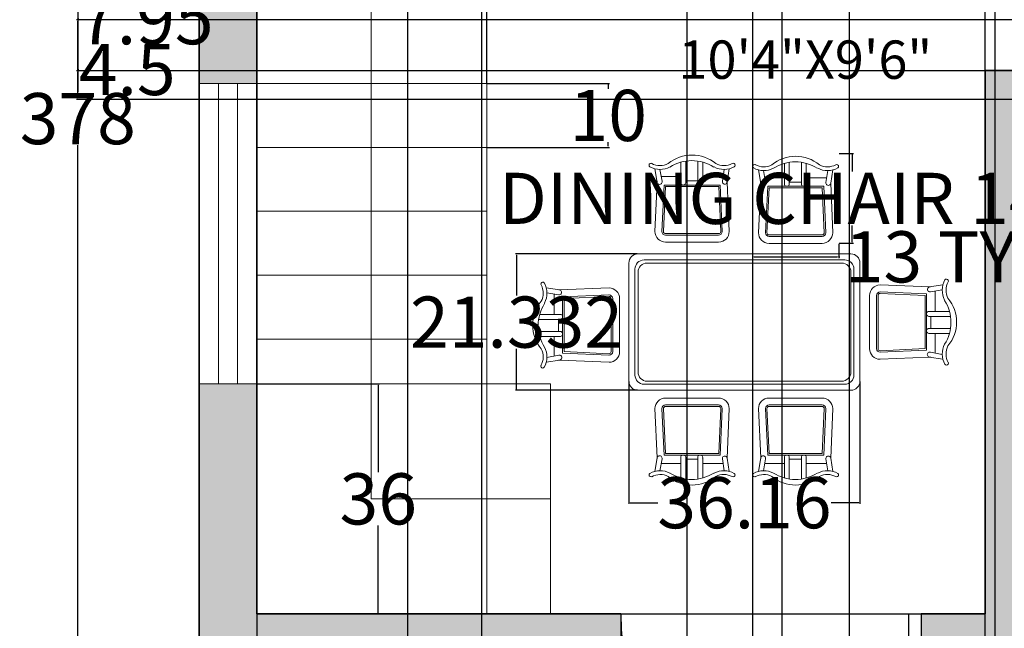
# Model space of a CAD drawing. Units: inches. Extents: x -24 to 368, y -370 to 58.
# Tile 2 of 9: x -24 to 130, y -235 to -140. Entities that reach past the tile are written whole.
import ezdxf

# ---------------------------------------------------------------- set-up
doc = ezdxf.new("R2010")
doc.units = ezdxf.units.IN
doc.header["$MEASUREMENT"] = 0
for name, color, linetype, lineweight in [('A-ANNO-DIMS', 2, 'Continuous', 18), ('A-AREA-IDEN', 7, 'Continuous', 18), ('A-FLOR-STRS', 7, 'Continuous', 18), ('A-WALL', 7, 'Continuous', 35), ('Furniture', 7, 'Continuous', 15)]:
    doc.layers.add(name, color=color, linetype=linetype, lineweight=lineweight)
for name, color, linetype, lineweight, true_color in [('A-DOOR', 40, 'Continuous', 25, 0xf8d731), ('A-GLAZ', 30, 'Continuous', 18, 0xf26722), ('A-WALL-PATT', 18, 'Continuous', 13, 0x000000)]:
    doc.layers.add(name, color=color, linetype=linetype, lineweight=lineweight, true_color=true_color)
doc.styles.get("Standard").update_dxf_attribs({"font": 'arial.ttf'})
doc.dimstyles.get("Standard").update_dxf_attribs({"dimtxt": 8, "dimasz": 0.18, "dimexe": 0.18, "dimexo": 0.0625, "dimgap": 0.09, "dimtad": 0, "dimtih": 1, "dimtoh": 1, "dimdec": 4, "dimzin": 0, "dimdsep": 46, "dimlunit": 3, "dimtxsty": 'Standard', "dimcen": 0.09, "dimclre": 5, "dimclrt": 6, "dimadec": 0, "dimazin": 0, "dimtfac": 1, "dimtdec": 4, "dimtofl": 0, "dimtmove": 0, "dimatfit": 3, "dimfxl": 1, "dimtolj": 1, "dimtzin": 0, "dimarcsym": 0})

# ---------------------------------------------------------------- blocks, each defined once
blk = doc.blocks.new('CHAIR-DINING')
for p, q in [((4.98, 9.38), (4.98, 12.51)), ((5.74, 9.38), (5.74, 12.67)), ((7.64, 12.68), (7.64, 9.38)), ((8.4, 12.52), (8.4, 9.39)), ((1.28, 9.34), (0.93, 11.48)), ((2.04, 9.52), (1.69, 11.38)), ((11.79, 11.38), (11.48, 9.52)), ((12.55, 11.48), (12.24, 9.4)), ((0.93, 1.66), (1.28, 9.34)), ((1.9, 10.25), (4.98, 10.25)), ((5.74, 9.59), (7.64, 9.59)), ((8.4, 10.25), (11.6, 10.25)), ((12.24, 9.4), (12.55, 1.66)), ((2.02, 1.67), (2.37, 8.93)), ((2.26, 1.66), (2.6, 8.69)), ((2.37, 8.93), (11.15, 8.93)), ((2.6, 8.69), (10.92, 8.69)), ((10.92, 8.69), (11.22, 1.66)), ((11.15, 8.93), (11.46, 1.67)), ((10.89, 1.33), (2.59, 1.33)), ((10.89, 1.09), (2.59, 1.09)), ((10.89, 0), (2.59, 0))]:
    blk.add_line(p, q)
for centre, radius, start, end in [((0.3, 12.04), 0.297, 56.5726, 237.7215), ((6.74, 7.78), 5.84, 50.3459, 129.6541), ((6.7, 6.41), 6.34, 57.3186, 122.6814), ((13.18, 12.04), 0.297, 302.2785, 123.4274), ((1.75, 14.71), 3.33, 241.1173, 297.5141), ((1.75, 14.71), 2.74, 240.9211, 297.5141), ((11.73, 14.71), 3.33, 242.4859, 298.8827), ((11.73, 14.71), 2.74, 242.4859, 298.022), ((1.66, 9.43), 0.39, 166.2748, 13.7252), ((5.36, 9.31), 0.387, 168.6748, 11.3252), ((8.02, 9.31), 0.387, 168.8014, 12.2085), ((11.86, 9.46), 0.384, 170.8614, 9.1386), ((2.59, 1.66), 1.66, 180, 270), ((2.59, 1.66), 0.569, 180, 270), ((2.59, 1.66), 0.332, 180, 270), ((10.89, 1.66), 1.66, 270, 0), ((10.89, 1.66), 0.569, 270, 0), ((10.89, 1.66), 0.332, 270, 0)]:
    blk.add_arc(centre, radius, start, end)
blk = doc.blocks.new('WINDOW-47')
for p, q in [((0, 47), (0, 0)), ((0, 47), (9, 47)), ((3, 47), (3, 0)), ((6, 47), (6, 0)), ((9, 0), (9, 47)), ((0, 0), (9, 0))]:
    blk.add_line(p, q)
blk = doc.blocks.new('DOOR-SINGLE-47')
for p, q in [((0, 0), (0, 47)), ((2, 0), (2, 47)), ((47, 0), (0, 0))]:
    blk.add_line(p, q)
blk.add_arc((0, 0), 47, 0, 90)
blk = doc.blocks.new('*D11')
at = {"layer": 'A-ANNO-DIMS', "color": 5, "lineweight": -2, "transparency": 16777216}
for p, q in [((104.31, -160.81), (106.54, -160.81)), ((104.31, -174.87), (106.54, -174.87))]:
    blk.add_line(p, q, dxfattribs=at)
at = {"layer": 'A-ANNO-DIMS', "color": 0, "lineweight": -2, "transparency": 16777216}
for p, q in [((106.36, -160.99), (106.36, -163.61)), ((106.36, -174.69), (106.36, -172.07))]:
    blk.add_line(p, q, dxfattribs=at)
at = {"layer": 'A-ANNO-DIMS', "color": 0, "transparency": 16777216}
for points in [[(106.33, -160.99), (106.39, -160.99), (106.36, -160.81)], [(106.33, -174.69), (106.39, -174.69), (106.36, -174.87)]]:
    blk.add_solid(points, dxfattribs=at)
at = {"layer": 'Defpoints', "color": 0, "transparency": 16777216}
for p in [(104.24, -160.81), (106.36, -160.81), (104.24, -174.87)]:
    blk.add_point(p, dxfattribs=at)
at = {"layer": 'A-ANNO-DIMS', "color": 6, "transparency": 16777216, "insert": (106.36, -167.84), "char_height": 8, "attachment_point": 5}
blk.add_mtext('\\A1;DINING CHAIR 14 TYP.', dxfattribs=at)
blk = doc.blocks.new('*D12')
at = {"layer": 'A-ANNO-DIMS', "color": 5, "lineweight": -2, "transparency": 16777216}
for p, q in [((90.76, -174.94), (90.76, -177.17)), ((104.24, -174.94), (104.24, -177.17))]:
    blk.add_line(p, q, dxfattribs=at)
at = {"layer": 'A-ANNO-DIMS', "color": 0, "lineweight": -2, "transparency": 16777216}
for p, q in [((90.94, -176.99), (104.06, -176.99)), ((104.24, -176.99), (104.42, -176.99))]:
    blk.add_line(p, q, dxfattribs=at)
at = {"layer": 'A-ANNO-DIMS', "color": 0, "transparency": 16777216}
for points in [[(90.94, -176.96), (90.94, -177.02), (90.76, -176.99)], [(104.06, -176.96), (104.06, -177.02), (104.24, -176.99)]]:
    blk.add_solid(points, dxfattribs=at)
at = {"layer": 'Defpoints', "color": 0, "transparency": 16777216}
for p in [(90.76, -174.87), (104.24, -174.87), (104.24, -176.99)]:
    blk.add_point(p, dxfattribs=at)
at = {"layer": 'A-ANNO-DIMS', "color": 6, "transparency": 16777216, "insert": (123.61, -176.99), "char_height": 8, "attachment_point": 5}
blk.add_mtext('\\A1;13 TYP.', dxfattribs=at)
blk = doc.blocks.new('*D26')
at = {"layer": 'A-ANNO-DIMS', "color": 5, "lineweight": -2, "transparency": 16777216}
for p, q in [((4.1, 33.64), (-15.03, 33.64)), ((4.1, -344.36), (-15.03, -344.36))]:
    blk.add_line(p, q, dxfattribs=at)
at = {"layer": 'A-ANNO-DIMS', "color": 0, "lineweight": -2, "transparency": 16777216}
for p, q in [((-14.85, 33.46), (-14.85, -151.18)), ((-14.85, -344.18), (-14.85, -159.53))]:
    blk.add_line(p, q, dxfattribs=at)
at = {"layer": 'A-ANNO-DIMS', "color": 0, "transparency": 16777216}
for points in [[(-14.88, 33.46), (-14.82, 33.46), (-14.85, 33.64)], [(-14.88, -344.18), (-14.82, -344.18), (-14.85, -344.36)]]:
    blk.add_solid(points, dxfattribs=at)
at = {"layer": 'Defpoints', "color": 0, "transparency": 16777216}
for p in [(-14.85, 33.64), (4.16, 33.64), (4.16, -344.36)]:
    blk.add_point(p, dxfattribs=at)
at = {"layer": 'A-ANNO-DIMS', "color": 6, "transparency": 16777216, "insert": (-14.85, -155.36), "char_height": 8, "attachment_point": 5}
blk.add_mtext('\\A1;378', dxfattribs=at)
blk = doc.blocks.new('*D40')
at = {"layer": 'A-ANNO-DIMS', "color": 5, "lineweight": -2, "transparency": 16777216}
for p, q in [((13.16, 24.58), (13.16, -363.55)), ((48.33, 24.58), (48.33, -363.55))]:
    blk.add_line(p, q, dxfattribs=at)
at = {"layer": 'A-ANNO-DIMS', "color": 0, "lineweight": -2, "transparency": 16777216}
for p, q in [((13.34, -363.37), (17.16, -363.37)), ((48.15, -363.37), (44.33, -363.37))]:
    blk.add_line(p, q, dxfattribs=at)
at = {"layer": 'A-ANNO-DIMS', "color": 0, "transparency": 16777216}
for points in [[(13.34, -363.34), (13.34, -363.4), (13.16, -363.37)], [(48.15, -363.34), (48.15, -363.4), (48.33, -363.37)]]:
    blk.add_solid(points, dxfattribs=at)
at = {"layer": 'Defpoints', "color": 0, "transparency": 16777216}
for p in [(13.16, 24.64), (48.33, 24.64), (48.33, -363.37)]:
    blk.add_point(p, dxfattribs=at)
at = {"layer": 'A-ANNO-DIMS', "color": 6, "transparency": 16777216, "insert": (30.75, -363.37), "char_height": 8, "attachment_point": 5}
blk.add_mtext('\\A1;35.17', dxfattribs=at)
blk = doc.blocks.new('*D41')
at = {"layer": 'A-ANNO-DIMS', "color": 5, "lineweight": -2, "transparency": 16777216}
for p, q in [((95.33, 24.58), (95.33, -363.55)), ((128.66, 24.58), (128.66, -363.55))]:
    blk.add_line(p, q, dxfattribs=at)
at = {"layer": 'A-ANNO-DIMS', "color": 0, "lineweight": -2, "transparency": 16777216}
for p, q in [((95.51, -363.37), (98.41, -363.37)), ((128.48, -363.37), (125.58, -363.37))]:
    blk.add_line(p, q, dxfattribs=at)
at = {"layer": 'A-ANNO-DIMS', "color": 0, "transparency": 16777216}
for points in [[(95.51, -363.34), (95.51, -363.4), (95.33, -363.37)], [(128.48, -363.34), (128.48, -363.4), (128.66, -363.37)]]:
    blk.add_solid(points, dxfattribs=at)
at = {"layer": 'Defpoints', "color": 0, "transparency": 16777216}
for p in [(95.33, 24.64), (128.66, 24.64), (128.66, -363.37)]:
    blk.add_point(p, dxfattribs=at)
at = {"layer": 'A-ANNO-DIMS', "color": 6, "transparency": 16777216, "insert": (112, -363.37), "char_height": 8, "attachment_point": 5}
blk.add_mtext('\\A1;33.33', dxfattribs=at)
blk = doc.blocks.new('*D45')
at = {"layer": 'A-ANNO-DIMS', "color": 5, "lineweight": -2, "transparency": 16777216}
for p, q in [((13.22, -196.86), (32.36, -196.86)), ((13.22, -232.86), (32.36, -232.86))]:
    blk.add_line(p, q, dxfattribs=at)
at = {"layer": 'A-ANNO-DIMS', "color": 0, "lineweight": -2, "transparency": 16777216}
for p, q in [((32.18, -197.04), (32.18, -210.68)), ((32.18, -232.68), (32.18, -219.03))]:
    blk.add_line(p, q, dxfattribs=at)
at = {"layer": 'A-ANNO-DIMS', "color": 0, "transparency": 16777216}
for points in [[(32.15, -197.04), (32.21, -197.04), (32.18, -196.86)], [(32.15, -232.68), (32.21, -232.68), (32.18, -232.86)]]:
    blk.add_solid(points, dxfattribs=at)
at = {"layer": 'Defpoints', "color": 0, "transparency": 16777216}
for p in [(13.16, -196.86), (13.16, -232.86), (32.18, -232.86)]:
    blk.add_point(p, dxfattribs=at)
at = {"layer": 'A-ANNO-DIMS', "color": 6, "transparency": 16777216, "insert": (32.18, -214.86), "char_height": 8, "attachment_point": 5}
blk.add_mtext('\\A1;36', dxfattribs=at)
blk = doc.blocks.new('*D47')
at = {"layer": 'A-ANNO-DIMS', "color": 5, "lineweight": -2, "transparency": 16777216}
for p, q in [((36.75, -58.62), (36.75, -363.55)), ((90.75, -58.62), (90.75, -363.55))]:
    blk.add_line(p, q, dxfattribs=at)
at = {"layer": 'A-ANNO-DIMS', "color": 0, "lineweight": -2, "transparency": 16777216}
for p, q in [((36.93, -363.37), (57.95, -363.37)), ((90.57, -363.37), (69.56, -363.37))]:
    blk.add_line(p, q, dxfattribs=at)
at = {"layer": 'A-ANNO-DIMS', "color": 0, "transparency": 16777216}
for points in [[(36.93, -363.34), (36.93, -363.4), (36.75, -363.37)], [(90.57, -363.34), (90.57, -363.4), (90.75, -363.37)]]:
    blk.add_solid(points, dxfattribs=at)
at = {"layer": 'Defpoints', "color": 0, "transparency": 16777216}
for p in [(36.75, -58.55), (90.75, -58.55), (90.75, -363.37)]:
    blk.add_point(p, dxfattribs=at)
at = {"layer": 'A-ANNO-DIMS', "color": 6, "transparency": 16777216, "insert": (63.75, -363.37), "char_height": 8, "attachment_point": 5}
blk.add_mtext('\\A1;54', dxfattribs=at)
blk = doc.blocks.new('*D49')
at = {"layer": 'A-ANNO-DIMS', "color": 5, "lineweight": -2, "transparency": 16777216}
for p, q in [((13.16, -149.79), (13.16, 52.85)), ((49.16, -149.79), (49.16, 52.85))]:
    blk.add_line(p, q, dxfattribs=at)
at = {"layer": 'A-ANNO-DIMS', "color": 0, "lineweight": -2, "transparency": 16777216}
for p, q in [((13.34, 52.67), (25.35, 52.67)), ((48.98, 52.67), (36.98, 52.67))]:
    blk.add_line(p, q, dxfattribs=at)
at = {"layer": 'A-ANNO-DIMS', "color": 0, "transparency": 16777216}
for points in [[(13.34, 52.7), (13.34, 52.64), (13.16, 52.67)], [(48.98, 52.7), (48.98, 52.64), (49.16, 52.67)]]:
    blk.add_solid(points, dxfattribs=at)
at = {"layer": 'Defpoints', "color": 0, "transparency": 16777216}
for p in [(49.16, 52.67), (13.16, -149.86), (49.16, -149.86)]:
    blk.add_point(p, dxfattribs=at)
at = {"layer": 'A-ANNO-DIMS', "color": 6, "transparency": 16777216, "insert": (31.16, 52.67), "char_height": 8, "attachment_point": 5}
blk.add_mtext('\\A1;36', dxfattribs=at)
blk = doc.blocks.new('*D50')
at = {"layer": 'A-ANNO-DIMS', "color": 5, "lineweight": -2, "transparency": 16777216}
for p, q in [((49.22, -149.86), (68.36, -149.86)), ((49.22, -159.86), (68.36, -159.86))]:
    blk.add_line(p, q, dxfattribs=at)
at = {"layer": 'A-ANNO-DIMS', "color": 0, "lineweight": -2, "transparency": 16777216}
for p, q in [((68.18, -150.04), (68.18, -150.68)), ((68.18, -159.68), (68.18, -159.03))]:
    blk.add_line(p, q, dxfattribs=at)
at = {"layer": 'A-ANNO-DIMS', "color": 0, "transparency": 16777216}
for points in [[(68.15, -150.04), (68.21, -150.04), (68.18, -149.86)], [(68.15, -159.68), (68.21, -159.68), (68.18, -159.86)]]:
    blk.add_solid(points, dxfattribs=at)
at = {"layer": 'Defpoints', "color": 0, "transparency": 16777216}
for p in [(49.16, -149.86), (49.16, -159.86), (68.18, -159.86)]:
    blk.add_point(p, dxfattribs=at)
at = {"layer": 'A-ANNO-DIMS', "color": 6, "transparency": 16777216, "insert": (68.18, -154.86), "char_height": 8, "attachment_point": 5}
blk.add_mtext('\\A1;10', dxfattribs=at)
blk = doc.blocks.new('*D53')
at = {"layer": 'A-ANNO-DIMS', "color": 5, "lineweight": -2, "transparency": 16777216}
for p, q in [((13.16, -89.42), (13.16, -363.55)), ((80.45, -89.42), (80.45, -363.55))]:
    blk.add_line(p, q, dxfattribs=at)
at = {"layer": 'A-ANNO-DIMS', "color": 0, "lineweight": -2, "transparency": 16777216}
for p, q in [((13.34, -363.37), (33.19, -363.37)), ((80.27, -363.37), (60.42, -363.37))]:
    blk.add_line(p, q, dxfattribs=at)
at = {"layer": 'A-ANNO-DIMS', "color": 0, "transparency": 16777216}
for points in [[(13.34, -363.34), (13.34, -363.4), (13.16, -363.37)], [(80.27, -363.34), (80.27, -363.4), (80.45, -363.37)]]:
    blk.add_solid(points, dxfattribs=at)
at = {"layer": 'Defpoints', "color": 0, "transparency": 16777216}
for p in [(13.16, -89.36), (80.45, -89.36), (80.45, -363.37)]:
    blk.add_point(p, dxfattribs=at)
at = {"layer": 'A-ANNO-DIMS', "color": 6, "transparency": 16777216, "insert": (46.81, -363.37), "char_height": 8, "attachment_point": 5}
blk.add_mtext('\\A1;67.29', dxfattribs=at)
blk = doc.blocks.new('*D54')
at = {"layer": 'A-ANNO-DIMS', "color": 5, "lineweight": -2, "transparency": 16777216}
for p, q in [((13.16, -232.92), (13.16, -363.55)), ((70.16, -232.92), (70.16, -363.55))]:
    blk.add_line(p, q, dxfattribs=at)
at = {"layer": 'A-ANNO-DIMS', "color": 0, "lineweight": -2, "transparency": 16777216}
for p, q in [((13.34, -363.37), (35.84, -363.37)), ((69.98, -363.37), (47.48, -363.37))]:
    blk.add_line(p, q, dxfattribs=at)
at = {"layer": 'A-ANNO-DIMS', "color": 0, "transparency": 16777216}
for points in [[(13.34, -363.34), (13.34, -363.4), (13.16, -363.37)], [(69.98, -363.34), (69.98, -363.4), (70.16, -363.37)]]:
    blk.add_solid(points, dxfattribs=at)
at = {"layer": 'Defpoints', "color": 0, "transparency": 16777216}
for p in [(13.16, -232.86), (70.16, -232.86), (70.16, -363.37)]:
    blk.add_point(p, dxfattribs=at)
at = {"layer": 'A-ANNO-DIMS', "color": 6, "transparency": 16777216, "insert": (41.66, -363.37), "char_height": 8, "attachment_point": 5}
blk.add_mtext('\\A1;57', dxfattribs=at)
blk = doc.blocks.new('*D57')
at = {"layer": 'A-ANNO-DIMS', "color": 5, "lineweight": -2, "transparency": 16777216}
for p, q in [((164.37, -147.86), (-15.03, -147.86)), ((164.37, -152.36), (-15.03, -152.36))]:
    blk.add_line(p, q, dxfattribs=at)
at = {"layer": 'A-ANNO-DIMS', "color": 0, "lineweight": -2, "transparency": 16777216}
for p, q in [((-14.85, -147.86), (-14.85, -147.68)), ((-14.85, -147.68), (-14.67, -147.68)), ((-14.85, -152.18), (-14.85, -148.04))]:
    blk.add_line(p, q, dxfattribs=at)
at = {"layer": 'A-ANNO-DIMS', "color": 0, "transparency": 16777216}
for points in [[(-14.88, -148.04), (-14.82, -148.04), (-14.85, -147.86)], [(-14.88, -152.18), (-14.82, -152.18), (-14.85, -152.36)]]:
    blk.add_solid(points, dxfattribs=at)
at = {"layer": 'Defpoints', "color": 0, "transparency": 16777216}
for p in [(-14.85, -147.86), (164.43, -147.86), (164.43, -152.36)]:
    blk.add_point(p, dxfattribs=at)
at = {"layer": 'A-ANNO-DIMS', "color": 6, "transparency": 16777216, "insert": (-7.11, -147.68), "char_height": 8, "attachment_point": 5}
blk.add_mtext('\\A1;4.5', dxfattribs=at)
blk = doc.blocks.new('*D59')
at = {"layer": 'A-ANNO-DIMS', "color": 5, "lineweight": -2, "transparency": 16777216}
for p, q in [((246.6, -139.91), (-15.03, -139.91)), ((246.6, -147.86), (-15.03, -147.86))]:
    blk.add_line(p, q, dxfattribs=at)
at = {"layer": 'A-ANNO-DIMS', "color": 0, "lineweight": -2, "transparency": 16777216}
for p, q in [((-14.85, -139.91), (-14.85, -139.73)), ((-14.85, -139.73), (-14.67, -139.73)), ((-14.85, -147.68), (-14.85, -140.09))]:
    blk.add_line(p, q, dxfattribs=at)
at = {"layer": 'A-ANNO-DIMS', "color": 0, "transparency": 16777216}
for points in [[(-14.88, -140.09), (-14.82, -140.09), (-14.85, -139.91)], [(-14.88, -147.68), (-14.82, -147.68), (-14.85, -147.86)]]:
    blk.add_solid(points, dxfattribs=at)
at = {"layer": 'Defpoints', "color": 0, "transparency": 16777216}
for p in [(-14.85, -139.91), (246.66, -139.91), (246.66, -147.86)]:
    blk.add_point(p, dxfattribs=at)
at = {"layer": 'A-ANNO-DIMS', "color": 6, "transparency": 16777216, "insert": (-4.2, -139.73), "char_height": 8, "attachment_point": 5}
blk.add_mtext('\\A1;7.95', dxfattribs=at)
blk = doc.blocks.new('*D65')
at = {"layer": 'A-ANNO-DIMS', "color": 5, "lineweight": -2, "transparency": 16777216}
for p, q in [((105.95, -335.29), (105.95, 52.85)), ((127.16, -335.29), (127.16, 52.85))]:
    blk.add_line(p, q, dxfattribs=at)
at = {"layer": 'A-ANNO-DIMS', "color": 0, "lineweight": -2, "transparency": 16777216}
for p, q in [((106.13, 52.67), (126.98, 52.67)), ((127.16, 52.67), (127.34, 52.67))]:
    blk.add_line(p, q, dxfattribs=at)
at = {"layer": 'A-ANNO-DIMS', "color": 0, "transparency": 16777216}
for points in [[(106.13, 52.7), (106.13, 52.64), (105.95, 52.67)], [(126.98, 52.7), (126.98, 52.64), (127.16, 52.67)]]:
    blk.add_solid(points, dxfattribs=at)
at = {"layer": 'Defpoints', "color": 0, "transparency": 16777216}
for p in [(127.16, 52.67), (105.95, -335.36), (127.16, -335.36)]:
    blk.add_point(p, dxfattribs=at)
at = {"layer": 'A-ANNO-DIMS', "color": 6, "transparency": 16777216, "insert": (140.23, 52.67), "char_height": 8, "attachment_point": 5}
blk.add_mtext('\\A1;21.21', dxfattribs=at)
blk = doc.blocks.new('*D68')
at = {"layer": 'A-ANNO-DIMS', "color": 5, "lineweight": -2, "transparency": 16777216}
for p, q in [((71.41, -196.5), (71.41, -215.64)), ((107.57, -196.5), (107.57, -215.64))]:
    blk.add_line(p, q, dxfattribs=at)
at = {"layer": 'A-ANNO-DIMS', "color": 0, "lineweight": -2, "transparency": 16777216}
for p, q in [((71.59, -215.46), (75.91, -215.46)), ((107.39, -215.46), (103.07, -215.46))]:
    blk.add_line(p, q, dxfattribs=at)
at = {"layer": 'A-ANNO-DIMS', "color": 0, "transparency": 16777216}
for points in [[(71.59, -215.43), (71.59, -215.49), (71.41, -215.46)], [(107.39, -215.43), (107.39, -215.49), (107.57, -215.46)]]:
    blk.add_solid(points, dxfattribs=at)
at = {"layer": 'Defpoints', "color": 0, "transparency": 16777216}
for p in [(71.41, -196.44), (107.57, -196.44), (71.41, -215.46)]:
    blk.add_point(p, dxfattribs=at)
at = {"layer": 'A-ANNO-DIMS', "color": 6, "transparency": 16777216, "insert": (89.49, -215.46), "char_height": 8, "attachment_point": 5}
blk.add_mtext('\\A1;36.16', dxfattribs=at)
blk = doc.blocks.new('*D69')
at = {"layer": 'A-ANNO-DIMS', "color": 5, "lineweight": -2, "transparency": 16777216}
for p, q in [((72.77, -176.53), (53.64, -176.53)), ((72.77, -197.86), (53.64, -197.86))]:
    blk.add_line(p, q, dxfattribs=at)
at = {"layer": 'A-ANNO-DIMS', "color": 0, "lineweight": -2, "transparency": 16777216}
for p, q in [((53.82, -176.71), (53.82, -183.02)), ((53.82, -197.68), (53.82, -191.38))]:
    blk.add_line(p, q, dxfattribs=at)
at = {"layer": 'A-ANNO-DIMS', "color": 0, "transparency": 16777216}
for points in [[(53.79, -176.71), (53.85, -176.71), (53.82, -176.53)], [(53.79, -197.68), (53.85, -197.68), (53.82, -197.86)]]:
    blk.add_solid(points, dxfattribs=at)
at = {"layer": 'Defpoints', "color": 0, "transparency": 16777216}
for p in [(53.82, -176.53), (72.83, -176.53), (72.83, -197.86)]:
    blk.add_point(p, dxfattribs=at)
at = {"layer": 'A-ANNO-DIMS', "color": 6, "transparency": 16777216, "insert": (53.82, -187.2), "char_height": 8, "attachment_point": 5}
blk.add_mtext('\\A1;21.332', dxfattribs=at)

msp = doc.modelspace()

# ---------------------------------------------------------------- hatches: boundary and pattern name
at = {"layer": 'A-WALL-PATT'}
h = msp.add_hatch(color=256, dxfattribs=at)
h.dxf.hatch_style = 1
h.paths.add_polyline_path([(13.1621, -93.8573), (80.4499, -93.8573), (80.4499, -89.3573), (13.1621, -89.3573), (13.1621, -61.0987), (4.1621, -61.0987), (4.1621, -149.8573), (13.1621, -149.8573)])
h.paths.add_polyline_path([(146.5668, -27.3573), (133.1621, -27.3573), (133.1621, 10.3323), (133.1272, 10.3313), (133.1621, 24.6427), (139.8141, 24.6427), (139.8141, 33.6427), (95.3329, 33.6427), (95.3329, 24.6427), (128.6621, 24.6427), (128.6621, -89.3573), (127.4499, -89.3573), (127.4499, -93.8573), (133.1621, -93.8573), (133.1621, -31.8573), (146.5668, -31.8573)])
h.paths.add_polyline_path([(197.6621, 24.6427), (236.2134, 24.6427), (236.2134, 33.6427), (169.8141, 33.6427), (169.8141, 24.6427), (193.1621, 24.6427), (193.1621, -27.3573), (181.5668, -27.3573), (181.5668, -31.8573), (193.1621, -31.8573), (193.1621, -95.8573), (199.2127, -95.8573), (199.2127, -91.3573), (197.6621, -91.3573)])
h.paths.add_polyline_path([(322.1621, -52.531), (313.1621, -52.531), (313.1621, -91.3573), (246.2127, -91.3573), (246.2127, -95.8573), (246.6621, -95.8573), (246.6621, -104.9077), (251.1621, -104.9077), (251.1621, -95.8573), (313.1621, -95.8573), (313.1621, -105.6922), (317.6621, -105.6922), (322.1621, -105.6922)])
h.paths.add_polyline_path([(322.1621, -135.6922), (313.1621, -135.6922), (313.1621, -147.8573), (251.1621, -147.8573), (251.1621, -139.9077), (246.6621, -139.9077), (246.6621, -147.8573), (199.43, -147.8573), (199.43, -152.3573), (313.1621, -152.3573), (313.1621, -194.6142), (317.6621, -194.6142), (322.1621, -194.6142)])
h.paths.add_polyline_path([(322.1621, -241.6142), (313.1621, -241.6142), (313.1621, -275.3573), (287.3912, -275.3573), (287.3912, -279.8573), (313.1621, -279.8573), (313.1621, -335.3573), (298.077, -335.3573), (298.077, -344.3573), (322.1621, -344.3573)])
h.paths.add_polyline_path([(263.077, -335.3573), (241.1621, -335.3573), (241.1621, -279.8573), (252.3912, -279.8573), (252.3912, -275.3573), (236.6621, -275.3573), (236.6621, -298.8573), (234.5689, -298.8573), (234.5689, -303.3573), (236.6621, -303.3573), (236.6621, -344.3573), (263.077, -344.3573), (263.077, -339.8573)])
h.paths.add_polyline_path([(175.5689, -298.8573), (131.6621, -298.8573), (131.6621, -152.3573), (164.43, -152.3573), (164.43, -147.8573), (127.1621, -147.8573), (127.1621, -232.8573), (117.1621, -232.8573), (117.1621, -237.3573), (127.1621, -237.3573), (127.1621, -335.3573), (84.4055, -335.3573), (84.4055, -344.3573), (131.6621, -344.3573), (131.6621, -303.3573), (175.5689, -303.3573)])
h.paths.add_polyline_path([(70.1621, -232.8573), (13.1621, -232.8573), (13.1621, -196.8573), (4.1621, -196.8573), (4.1621, -257.9061), (13.1621, -257.9061), (13.1621, -237.3573), (70.1621, -237.3573)])
h.paths.add_polyline_path([(13.1621, -304.9061), (4.1621, -304.9061), (4.1621, -344.3573), (37.4055, -344.3573), (37.4055, -335.3573), (13.1621, -335.3573)])
h.paths.add_polyline_path([(322.1621, 33.6427), (283.2134, 33.6427), (283.2134, 24.6427), (313.1621, 24.6427), (313.1621, 11.9273), (313.4656, 11.629), (313.1621, 11.629), (313.1621, -5.531), (322.1621, -5.531)])
h.paths.add_polyline_path([(48.3329, 33.6427), (4.1621, 33.6427), (4.1621, -14.0987), (13.1621, -14.0987), (13.1621, 24.6427), (48.3329, 24.6427)])

# ---------------------------------------------------------------- linework, layer by layer
at = {"layer": 'A-DOOR'}
for p, q in [((70.1621, -232.8573), (70.1621, -237.3573)), ((117.1621, -232.8573), (117.1621, -237.3573))]:
    msp.add_line(p, q, dxfattribs=at)
at = {"layer": 'A-FLOR-STRS'}
for p, q in [((49.1621, -232.8573), (49.1621, -93.8573)), ((31.0603, -214.8573), (31.0603, -113.8048)), ((13.1621, -149.8573), (49.1621, -149.8573)), ((13.1621, -159.8573), (49.1621, -159.8573)), ((13.1621, -169.8573), (49.1621, -169.8573)), ((13.1621, -179.8573), (49.1621, -179.8573)), ((13.1621, -189.8573), (49.1621, -189.8573)), ((59.1621, -196.8573), (13.1621, -196.8573)), ((59.1621, -232.8573), (59.1621, -196.8573)), ((59.1621, -214.8573), (31.0603, -214.8573))]:
    msp.add_line(p, q, dxfattribs=at)
at = {"layer": 'A-WALL'}
for p, q in [((4.1621, -344.3573), (4.1621, 33.6427)), ((13.1621, -232.8573), (13.1621, -93.8573)), ((127.1621, -147.8573), (164.43, -147.8573)), ((127.1621, -232.8573), (127.1621, -147.8573)), ((70.1621, -232.8573), (13.1621, -232.8573)), ((127.1621, -232.8573), (117.1621, -232.8573))]:
    msp.add_line(p, q, dxfattribs=at)
at = {"layer": 'Furniture'}
for p, q in [((72.8319, -176.5324), (89.4897, -176.5324)), ((89.4897, -176.5324), (106.1475, -176.5324)), ((71.4097, -187.1985), (71.4097, -177.9546)), ((73.78, -177.4805), (89.4897, -177.4805)), ((74.254, -177.9546), (89.4897, -177.9546)), ((89.4897, -177.4805), (105.1994, -177.4805)), ((89.4897, -177.9546), (104.7253, -177.9546)), ((107.5696, -177.9546), (107.5696, -187.1985)), ((72.3578, -187.1985), (72.3578, -178.9027)), ((72.8319, -187.1985), (72.8319, -179.3767)), ((106.1475, -179.3767), (106.1475, -187.1985)), ((106.6215, -178.9027), (106.6215, -187.1985)), ((71.4097, -187.1985), (71.4097, -196.4425)), ((72.3578, -187.1985), (72.3578, -195.4944)), ((72.8319, -187.1985), (72.8319, -195.0204)), ((106.1475, -195.0204), (106.1475, -187.1985)), ((106.6215, -195.4944), (106.6215, -187.1985)), ((107.5696, -196.4425), (107.5696, -187.1985)), ((73.78, -196.9165), (89.4897, -196.9165)), ((74.254, -196.4425), (89.4897, -196.4425)), ((89.4897, -196.4425), (104.7253, -196.4425)), ((89.4897, -196.9165), (105.1994, -196.9165)), ((72.8319, -197.8646), (89.4897, -197.8646)), ((89.4897, -197.8646), (106.1475, -197.8646))]:
    msp.add_line(p, q, dxfattribs=at)
for centre, start, end in [((72.8319, -177.9546), 90, 180), ((106.1475, -177.9546), 0, 90), ((73.78, -178.9027), 90, 180), ((74.254, -179.3767), 90, 180), ((104.7253, -179.3767), 0, 90), ((105.1994, -178.9027), 0, 90), ((73.78, -195.4944), 180, 270), ((74.254, -195.0204), 180, 270), ((104.7253, -195.0204), 270, 0), ((105.1994, -195.4944), 270, 0), ((72.8319, -196.4425), 180, 270), ((106.1475, -196.4425), 270, 0)]:
    msp.add_arc(centre, 1.4221, start, end, dxfattribs=at)

# ---------------------------------------------------------------- block references
at = {"layer": 'A-DOOR', "rotation": 180}
msp.add_blockref('DOOR-SINGLE-47', (117.1618, -232.8576), dxfattribs=at)
at = {"layer": 'A-GLAZ'}
msp.add_blockref('WINDOW-47', (4.162, -196.8572), dxfattribs=at)
at = {"layer": 'Furniture'}
for p in [(74.553, -174.684), (90.7605, -174.8748)]:
    msp.add_blockref('CHAIR-DINING', p, dxfattribs=at)
at = {"layer": 'Furniture', "rotation": 89.99999999996653}
msp.add_blockref('CHAIR-DINING', (69.9593, -194.4084), dxfattribs=at)
at = {"layer": 'Furniture', "extrusion": (0, 0, -1), "zscale": -1}
for p, rotation in [((-109.0678, -193.9383), 89.99999999994922), ((-74.553, -199.074), 180), ((-90.7605, -199.074), 180)]:
    msp.add_blockref('CHAIR-DINING', p, dxfattribs=dict(at, rotation=rotation))

# ---------------------------------------------------------------- texts
at = {"layer": 'A-AREA-IDEN'}
msp.add_text('10\'4"X9\'6"', height=6, dxfattribs=at).set_placement((79.1621, -149.1343))
at = {"layer": 'Furniture', "flags": 9}
for tag, s in [('YSIZE', '2019.3631'), ('XSIZE', '1591.9460'), ('ZSIZE', '0.0429')]:
    msp.add_attdef(tag, (87.5924, -186.9923), s, height=0.01646, rotation=270, dxfattribs=at)

# ---------------------------------------------------------------- dimensions: what is measured, and where the dimension line sits
at = {"layer": 'A-ANNO-DIMS'}
for base, p1, p2, override, picture, middle in [((49.1621, 52.6658), (13.1621, -149.8573), (49.1621, -149.8573), {"dimdec": 0, "dimlfac": 1, "dimrnd": 0, "dimzin": 0, "dimdsep": 46, "dimlunit": 2}, '*D49', (31.1621, 52.6658)), ((127.1621, 52.6658), (105.953, -335.3573), (127.1621, -335.3573), {"dimdec": 2, "dimlfac": 1, "dimrnd": 0, "dimzin": 0, "dimdsep": 46, "dimlunit": 2}, '*D65', (140.2261, 52.6658)), ((48.3329, -363.3723), (13.1621, 24.6427), (48.3329, 24.6427), {"dimdec": 2, "dimlfac": 1, "dimrnd": 0, "dimzin": 0, "dimdsep": 46, "dimlunit": 2}, '*D40', (30.7475, -363.3723)), ((128.6621, -363.3723), (95.3329, 24.6427), (128.6621, 24.6427), {"dimdec": 2, "dimlfac": 1, "dimrnd": 0, "dimzin": 0, "dimdsep": 46, "dimlunit": 2}, '*D41', (111.9975, -363.3723)), ((90.7545, -363.3723), (36.7545, -58.5547), (90.7545, -58.5547), {"dimdec": 0, "dimlfac": 1, "dimrnd": 0, "dimzin": 0, "dimdsep": 46, "dimlunit": 2}, '*D47', (63.7545, -363.3723)), ((80.4499, -363.3723), (13.1621, -89.3573), (80.4499, -89.3573), {"dimdec": 2, "dimlfac": 1, "dimrnd": 0, "dimzin": 0, "dimdsep": 46, "dimlunit": 2}, '*D53', (46.806, -363.3723)), ((70.1621, -363.3723), (13.1621, -232.8573), (70.1621, -232.8573), {"dimdec": 0, "dimlfac": 1, "dimrnd": 0, "dimzin": 0, "dimdsep": 46, "dimlunit": 2}, '*D54', (41.6621, -363.3723))]:
    dim = msp.add_linear_dim(base=base, p1=p1, p2=p2, dimstyle='Standard', override=override, dxfattribs=at)
    dim.commit()
    dim.dimension.update_dxf_attribs({"geometry": picture, "text_midpoint": middle})
for base, p1, p2, angle, override, picture, middle in [((-14.8529, 33.6427), (4.1621, -344.3573), (4.1621, 33.6427), 90, {"dimdec": 0, "dimlfac": 1, "dimrnd": 0, "dimzin": 0, "dimdsep": 46, "dimlunit": 2}, '*D26', (-14.8529, -155.3573)), ((-14.8529, -139.9077), (246.6621, -147.8573), (246.6621, -139.9077), 90, {"dimdec": 2, "dimlfac": 1, "dimrnd": 0, "dimzin": 0, "dimdsep": 46, "dimlunit": 2}, '*D59', (-4.1955, -139.7277)), ((-14.8529, -147.8573), (164.43, -152.3573), (164.43, -147.8573), 90, {"dimdec": 1, "dimlfac": 1, "dimrnd": 0, "dimzin": 0, "dimdsep": 46, "dimlunit": 2}, '*D57', (-7.1095, -147.6773)), ((68.1771, -159.8573), (49.1621, -149.8573), (49.1621, -159.8573), 270, {"dimdec": 0, "dimlfac": 1, "dimrnd": 0, "dimzin": 0, "dimdsep": 46, "dimlunit": 2}, '*D50', (68.1771, -154.8573)), ((53.8169, -176.5324), (72.8319, -197.8646), (72.8319, -176.5324), 90, {"dimdec": 3, "dimlfac": 1, "dimrnd": 0, "dimzin": 0, "dimdsep": 46, "dimlunit": 2}, '*D69', (53.8169, -187.1985)), ((32.1771, -232.8573), (13.1621, -196.8573), (13.1621, -232.8573), 270, {"dimdec": 0, "dimlfac": 1, "dimrnd": 0, "dimzin": 0, "dimdsep": 46, "dimlunit": 2}, '*D45', (32.1771, -214.8573)), ((71.4097, -215.4575), (107.5696, -196.4425), (71.4097, -196.4425), 180, {"dimdec": 2, "dimlfac": 1, "dimrnd": 0, "dimzin": 0, "dimdsep": 46, "dimlunit": 2}, '*D68', (89.4897, -215.4575))]:
    dim = msp.add_linear_dim(base=base, p1=p1, p2=p2, angle=angle, dimstyle='Standard', override=override, dxfattribs=at)
    dim.commit()
    dim.dimension.update_dxf_attribs({"geometry": picture, "text_midpoint": middle})
dim = msp.add_linear_dim(base=(106.3552, -160.806), p1=(104.2448, -174.8749), p2=(104.2448, -160.806), angle=90, text='DINING CHAIR <> TYP.', dimstyle='Standard', override={"dimdec": 0, "dimlfac": 1, "dimrnd": 0, "dimzin": 0, "dimdsep": 46, "dimlunit": 2}, dxfattribs=at)
dim.commit()
dim.dimension.update_dxf_attribs({"geometry": '*D11', "text_midpoint": (106.3552, -167.8404)})
dim = msp.add_linear_dim(base=(104.2448, -176.9852), p1=(90.7557, -174.8749), p2=(104.2448, -174.8749), text='<> TYP.', dimstyle='Standard', override={"dimdec": 0, "dimlfac": 1, "dimrnd": 0, "dimzin": 0, "dimdsep": 46, "dimlunit": 2}, dxfattribs=at)
dim.commit()
dim.dimension.update_dxf_attribs({"geometry": '*D12', "text_midpoint": (123.609, -176.9852)})

doc.saveas('drawing.dxf')
